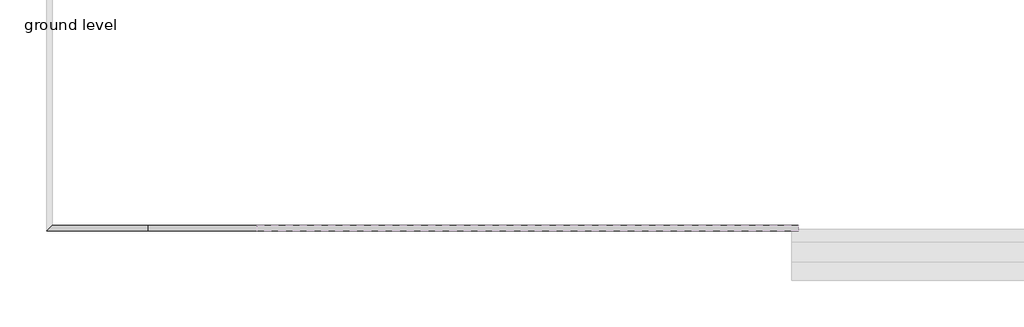
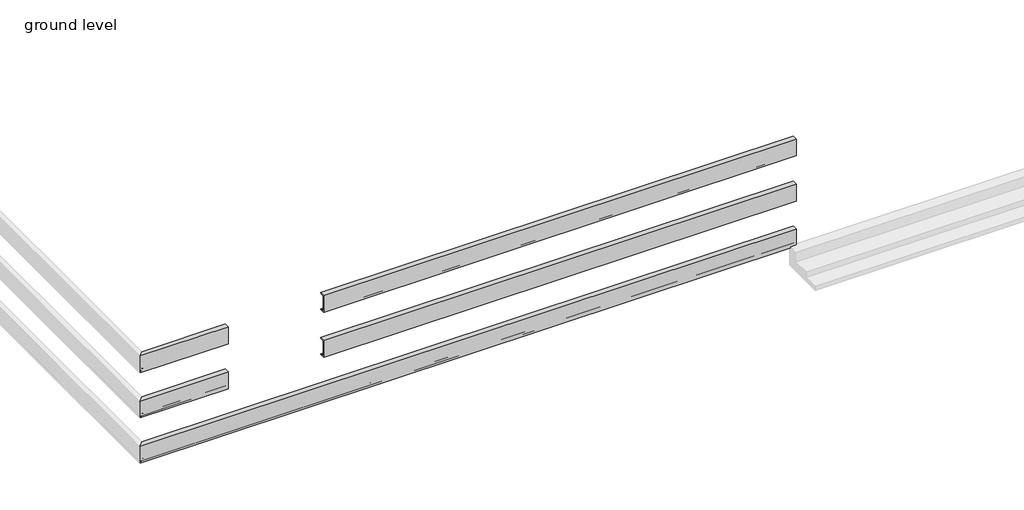
# One storey, part 1 of 3: 3 proxies.
"""IFC4 building model written with IfcOpenShell, lengths in millimetres."""

from ifc_helpers import new_model, si_unit, frame, origin, place, context, project, spatial, polyline, circle_curve, ellipse_curve, element, save
from ifc_brep_helpers import plane_surface, cylinder_surface, revolved_surface, advanced_brep

model = new_model("IFC4")

# Units and contexts
model_context = context("Model", 3, world=origin())
ifc_project = project(units=[si_unit("LENGTHUNIT", "METRE", prefix="MILLI")], contexts=[model_context])

# Site, building, storey
site = spatial("IfcSite", under=ifc_project)
building = spatial("IfcBuilding", under=site)
storey = spatial("IfcBuildingStorey", under=building, Name="ground level", Elevation=0.0)

# Proxies
placement = place(None, origin())
element("IfcBuildingElementProxy", 1, Name="Reveal", ObjectType="Reveal", at=placement, inside=storey, context=model_context, shape_type="AdvancedBrep", body=[
    advanced_brep(
    [(-10842.2672301, -7280.1146427, 1689.1), (-10842.2672301, -7216.8686427, 1689.1), (-10842.2672301, -7216.8686427, 1687.7203242), (-10842.2672301, -7221.2514519, 1682.5465897), (-10842.2672301, -7244.8721427, 1678.6098), (-10842.2672301, -7264.1100243, 1675.40348), (-10842.2672301, -7272.8756427, 1665.056011), (-10842.2672301, -7272.8756427, 1484.543989), (-10842.2672301, -7264.1100243, 1474.19652), (-10842.2672301, -7244.8721427, 1470.9902), (-10842.2672301, -7221.2514519, 1467.0534103), (-10842.2672301, -7216.8686427, 1461.8796758), (-10842.2672301, -7216.8686427, 1460.5), (-10842.2672301, -7280.1146427, 1460.5), (-4797.0672301, -7280.1146427, 1689.1), (-4797.0672301, -7280.1146427, 1460.5), (-4797.0672301, -7216.8686427, 1460.5), (-4797.0672301, -7216.8686427, 1461.8796758), (-4797.0672301, -7221.2514519, 1467.0534103), (-4797.0672301, -7244.8721427, 1470.9902), (-4797.0672301, -7264.1100243, 1474.19652), (-4797.0672301, -7272.8756427, 1484.543989), (-4797.0672301, -7272.8756427, 1665.056011), (-4797.0672301, -7264.1100243, 1675.40348), (-4797.0672301, -7244.8721427, 1678.6098), (-4797.0672301, -7221.2514519, 1682.5465897), (-4797.0672301, -7216.8686427, 1687.7203242), (-4797.0672301, -7216.8686427, 1689.1)],
    [
        (0, 1),
        (1, 2),
        (2, 3, circle_curve(frame((-10842.2672301, -7222.1137427, 1687.7203242), z_axis=(-1.0, 0.0, 0.0), x_axis=(0.0, 1.0, 0.0)), 5.2451)),
        (3, 4),
        (4, 5),
        (5, 6, circle_curve(frame((-10842.2672301, -7262.3854427, 1665.056011), z_axis=(1.0, 0.0, 0.0), x_axis=(0.0, 1.0, 0.0)), 10.4902)),
        (6, 7),
        (7, 8, circle_curve(frame((-10842.2672301, -7262.3854427, 1484.543989), z_axis=(1.0, 0.0, 0.0), x_axis=(0.0, 1.0, 0.0)), 10.4902)),
        (8, 9),
        (9, 10),
        (10, 11, circle_curve(frame((-10842.2672301, -7222.1137427, 1461.8796758), z_axis=(-1.0, 0.0, 0.0), x_axis=(0.0, 1.0, 0.0)), 5.2451)),
        (11, 12),
        (12, 13),
        (13, 0),
        (14, 15),
        (15, 16),
        (16, 17),
        (17, 18, circle_curve(frame((-4797.0672301, -7222.1137427, 1461.8796758), z_axis=(1.0, 0.0, 0.0), x_axis=(0.0, 1.0, 0.0)), 5.2451)),
        (18, 19),
        (19, 20),
        (20, 21, circle_curve(frame((-4797.0672301, -7262.3854427, 1484.543989), z_axis=(-1.0, 0.0, 0.0), x_axis=(0.0, 1.0, 0.0)), 10.4902)),
        (21, 22),
        (22, 23, circle_curve(frame((-4797.0672301, -7262.3854427, 1665.056011), z_axis=(-1.0, 0.0, 0.0), x_axis=(0.0, 1.0, 0.0)), 10.4902)),
        (23, 24),
        (24, 25),
        (25, 26, circle_curve(frame((-4797.0672301, -7222.1137427, 1687.7203242), z_axis=(1.0, 0.0, 0.0), x_axis=(0.0, 1.0, 0.0)), 5.2451)),
        (26, 27),
        (27, 14),
        (0, 14),
        (27, 1),
        (26, 2),
        (25, 3),
        (24, 4),
        (23, 5),
        (22, 6),
        (21, 7),
        (20, 8),
        (19, 9),
        (18, 10),
        (17, 11),
        (16, 12),
        (15, 13),
    ],
    [
        plane_surface(frame((-10842.2672301, -7036.6302427, 914.4), z_axis=(-1.0, 0.0, 0.0), x_axis=(0.0, -1.0, 0.0))),
        plane_surface(frame((-4797.0672301, -7265.2302427, 1450.6898298), z_axis=(1.0, 0.0, 0.0), x_axis=(0.0, 1.0, 0.0))),
        plane_surface(frame((-10842.2672301, -7280.1146427, 1689.1), z_axis=(0.0, 0.0, 1.0), x_axis=(1.0, 0.0, 0.0))),
        plane_surface(frame((-10842.2672301, -7216.8686427, 1689.1), z_axis=(0.0, 1.0, 0.0), x_axis=(1.0, 0.0, 0.0))),
        cylinder_surface(frame((-10842.2672301, -7222.1137427, 1687.7203242), z_axis=(-1.0, 0.0, 0.0), x_axis=(0.0, 1.0, 0.0)), 5.2451),
        plane_surface(frame((-10842.2672301, -7221.2514519, 1682.5465897), z_axis=(0.0, 0.16439930721687082, -0.9863938705135049), x_axis=(1.0, 0.0, 0.0))),
        plane_surface(frame((-10842.2672301, -7244.8721427, 1678.6098), z_axis=(0.0, 0.16439930721687146, -0.9863938705135048), x_axis=(1.0, 0.0, 0.0))),
        revolved_surface(polyline([(-4797.0672301, -7251.8952426999995, 1665.056011), (-10842.2672301, -7251.8952426999995, 1665.056011)]), (-10842.2672301, -7262.3854427, 1665.056011), (1.0, 0.0, 0.0)),
        plane_surface(frame((-10842.2672301, -7272.8756427, 1665.056011), z_axis=(0.0, 1.0, 0.0), x_axis=(1.0, 0.0, 0.0))),
        revolved_surface(polyline([(-4797.0672301, -7251.8952426999995, 1484.543989), (-10842.2672301, -7251.8952426999995, 1484.543989)]), (-10842.2672301, -7262.3854427, 1484.543989), (1.0, 0.0, 0.0)),
        plane_surface(frame((-10842.2672301, -7264.1100243, 1474.19652), z_axis=(0.0, 0.1643993072168769, 0.9863938705135039), x_axis=(1.0, 0.0, 0.0))),
        plane_surface(frame((-10842.2672301, -7244.8721427, 1470.9902), z_axis=(0.0, 0.16439930721687793, 0.9863938705135037), x_axis=(1.0, 0.0, 0.0))),
        cylinder_surface(frame((-10842.2672301, -7222.1137427, 1461.8796758), z_axis=(-1.0, 0.0, 0.0), x_axis=(0.0, 1.0, 0.0)), 5.2451),
        plane_surface(frame((-10842.2672301, -7216.8686427, 1461.8796758), z_axis=(0.0, 1.0, 0.0), x_axis=(1.0, 0.0, 0.0))),
        plane_surface(frame((-10842.2672301, -7216.8686427, 1460.5), z_axis=(0.0, 0.0, -1.0), x_axis=(1.0, 0.0, 0.0))),
        plane_surface(frame((-10842.2672301, -7280.1146427, 1460.5), z_axis=(0.0, -1.0, 0.0), x_axis=(1.0, 0.0, 0.0))),
    ],
    [
        (0, [[1, 2, 3, 4, 5, 6, 7, 8, 9, 10, 11, 12, 13, 14]]),
        (1, [[15, 16, 17, 18, 19, 20, 21, 22, 23, 24, 25, 26, 27, 28]]),
        (2, [[-1, 29, -28, 30]]),
        (3, [[-2, -30, -27, 31]]),
        (4, [[-3, -31, -26, 32]]),
        (5, [[-4, -32, -25, 33]]),
        (6, [[-5, -33, -24, 34]]),
        (7, [[-6, -34, -23, 35]]),
        (8, [[-7, -35, -22, 36]]),
        (9, [[-8, -36, -21, 37]]),
        (10, [[-9, -37, -20, 38]]),
        (11, [[-10, -38, -19, 39]]),
        (12, [[-11, -39, -18, 40]]),
        (13, [[-12, -40, -17, 41]]),
        (14, [[-13, -41, -16, 42]]),
        (15, [[-14, -42, -15, -29]]),
    ],
),
    advanced_brep(
    [(-13193.9516301, -7280.1146427, 1689.1), (-13130.7056301, -7216.8686427, 1689.1), (-13130.7056301, -7216.8686427, 1687.7203242), (-13135.0884393, -7221.2514519, 1682.5465897), (-13158.7091301, -7244.8721427, 1678.6098), (-13177.9470117, -7264.1100243, 1675.40348), (-13186.7126301, -7272.8756427, 1665.056011), (-13186.7126301, -7272.8756427, 1484.543989), (-13177.9470117, -7264.1100243, 1474.19652), (-13158.7091301, -7244.8721427, 1470.9902), (-13135.0884393, -7221.2514519, 1467.0534103), (-13130.7056301, -7216.8686427, 1461.8796758), (-13130.7056301, -7216.8686427, 1460.5), (-13193.9516301, -7280.1146427, 1460.5), (-12061.4672301, -7280.1146427, 1689.1), (-12061.4672301, -7280.1146427, 1460.5), (-12061.4672301, -7216.8686427, 1460.5), (-12061.4672301, -7216.8686427, 1461.8796758), (-12061.4672301, -7221.2514519, 1467.0534103), (-12061.4672301, -7244.8721427, 1470.9902), (-12061.4672301, -7264.1100243, 1474.19652), (-12061.4672301, -7272.8756427, 1484.543989), (-12061.4672301, -7272.8756427, 1665.056011), (-12061.4672301, -7264.1100243, 1675.40348), (-12061.4672301, -7244.8721427, 1678.6098), (-12061.4672301, -7221.2514519, 1682.5465897), (-12061.4672301, -7216.8686427, 1687.7203242), (-12061.4672301, -7216.8686427, 1689.1)],
    [
        (0, 1),
        (1, 2),
        (2, 3, ellipse_curve(frame((-13135.9507301, -7222.1137427, 1687.7203242), z_axis=(-0.7071067811865476, 0.7071067811865476, 0.0), x_axis=(-0.7071067811865475, -0.7071067811865476, 0.0)), 7.4176916, 5.2451)),
        (3, 4),
        (4, 5),
        (5, 6, ellipse_curve(frame((-13176.2224301, -7262.3854427, 1665.056011), z_axis=(0.7071067811865476, -0.7071067811865476, 0.0), x_axis=(0.7071067811865475, 0.7071067811865476, 0.0)), 14.8353831, 10.4902)),
        (6, 7),
        (7, 8, ellipse_curve(frame((-13176.2224301, -7262.3854427, 1484.543989), z_axis=(0.7071067811865476, -0.7071067811865476, 0.0), x_axis=(0.7071067811865475, 0.7071067811865476, 0.0)), 14.8353831, 10.4902)),
        (8, 9),
        (9, 10),
        (10, 11, ellipse_curve(frame((-13135.9507301, -7222.1137427, 1461.8796758), z_axis=(-0.7071067811865476, 0.7071067811865476, 0.0), x_axis=(-0.7071067811865475, -0.7071067811865476, 0.0)), 7.4176916, 5.2451)),
        (11, 12),
        (12, 13),
        (13, 0),
        (14, 15),
        (15, 16),
        (16, 17),
        (17, 18, circle_curve(frame((-12061.4672301, -7222.1137427, 1461.8796758), z_axis=(1.0, 0.0, 0.0), x_axis=(0.0, 1.0, 0.0)), 5.2451)),
        (18, 19),
        (19, 20),
        (20, 21, circle_curve(frame((-12061.4672301, -7262.3854427, 1484.543989), z_axis=(-1.0, 0.0, 0.0), x_axis=(0.0, 1.0, 0.0)), 10.4902)),
        (21, 22),
        (22, 23, circle_curve(frame((-12061.4672301, -7262.3854427, 1665.056011), z_axis=(-1.0, 0.0, 0.0), x_axis=(0.0, 1.0, 0.0)), 10.4902)),
        (23, 24),
        (24, 25),
        (25, 26, circle_curve(frame((-12061.4672301, -7222.1137427, 1687.7203242), z_axis=(1.0, 0.0, 0.0), x_axis=(0.0, 1.0, 0.0)), 5.2451)),
        (26, 27),
        (27, 14),
        (0, 14),
        (27, 1),
        (26, 2),
        (25, 3),
        (24, 4),
        (23, 5),
        (22, 6),
        (21, 7),
        (20, 8),
        (19, 9),
        (18, 10),
        (17, 11),
        (16, 12),
        (15, 13),
    ],
    [
        plane_surface(frame((-13179.0672301, -7265.2302427, 1270.0), z_axis=(-0.7071067811865476, 0.7071067811865476, 0.0), x_axis=(0.7071067811865476, 0.7071067811865476, 0.0))),
        plane_surface(frame((-12061.4672301, -7036.6302427, 2184.4), z_axis=(1.0, 0.0, 0.0), x_axis=(0.0, -1.0, 0.0))),
        plane_surface(frame((-13193.9516301, -7280.1146427, 1689.1), z_axis=(0.0, 0.0, 1.0), x_axis=(1.0, 0.0, 0.0))),
        plane_surface(frame((-13130.7056301, -7216.8686427, 1689.1), z_axis=(0.0, 1.0, 0.0), x_axis=(1.0, 0.0, 0.0))),
        cylinder_surface(frame((-13179.0672301, -7222.1137427, 1687.7203242), z_axis=(-1.0, 0.0, 0.0), x_axis=(0.0, 1.0, 0.0)), 5.2451),
        plane_surface(frame((-13135.0884393, -7221.2514519, 1682.5465897), z_axis=(0.0, 0.16439930721687082, -0.9863938705135049), x_axis=(1.0, 0.0, 0.0))),
        plane_surface(frame((-13158.7091301, -7244.8721427, 1678.6098), z_axis=(0.0, 0.16439930721687146, -0.9863938705135048), x_axis=(1.0, 0.0, 0.0))),
        revolved_surface(polyline([(-12061.4672301, -7251.8952426999995, 1665.056011), (-13186.7126301, -7251.8952426999995, 1665.056011)]), (-13179.0672301, -7262.3854427, 1665.056011), (1.0, 0.0, 0.0)),
        plane_surface(frame((-13186.7126301, -7272.8756427, 1665.056011), z_axis=(0.0, 1.0, 0.0), x_axis=(1.0, 0.0, 0.0))),
        revolved_surface(polyline([(-12061.4672301, -7251.8952426999995, 1484.543989), (-13186.7126301, -7251.8952426999995, 1484.543989)]), (-13179.0672301, -7262.3854427, 1484.543989), (1.0, 0.0, 0.0)),
        plane_surface(frame((-13177.9470117, -7264.1100243, 1474.19652), z_axis=(0.0, 0.1643993072168769, 0.9863938705135039), x_axis=(1.0, 0.0, 0.0))),
        plane_surface(frame((-13158.7091301, -7244.8721427, 1470.9902), z_axis=(0.0, 0.16439930721687793, 0.9863938705135037), x_axis=(1.0, 0.0, 0.0))),
        cylinder_surface(frame((-13179.0672301, -7222.1137427, 1461.8796758), z_axis=(-1.0, 0.0, 0.0), x_axis=(0.0, 1.0, 0.0)), 5.2451),
        plane_surface(frame((-13130.7056301, -7216.8686427, 1461.8796758), z_axis=(0.0, 1.0, 0.0), x_axis=(1.0, 0.0, 0.0))),
        plane_surface(frame((-13130.7056301, -7216.8686427, 1460.5), z_axis=(0.0, 0.0, -1.0), x_axis=(1.0, 0.0, 0.0))),
        plane_surface(frame((-13193.9516301, -7280.1146427, 1460.5), z_axis=(0.0, -1.0, 0.0), x_axis=(1.0, 0.0, 0.0))),
    ],
    [
        (0, [[1, 2, 3, 4, 5, 6, 7, 8, 9, 10, 11, 12, 13, 14]]),
        (1, [[15, 16, 17, 18, 19, 20, 21, 22, 23, 24, 25, 26, 27, 28]]),
        (2, [[-1, 29, -28, 30]]),
        (3, [[-2, -30, -27, 31]]),
        (4, [[-3, -31, -26, 32]]),
        (5, [[-4, -32, -25, 33]]),
        (6, [[-5, -33, -24, 34]]),
        (7, [[-6, -34, -23, 35]]),
        (8, [[-7, -35, -22, 36]]),
        (9, [[-8, -36, -21, 37]]),
        (10, [[-9, -37, -20, 38]]),
        (11, [[-10, -38, -19, 39]]),
        (12, [[-11, -39, -18, 40]]),
        (13, [[-12, -40, -17, 41]]),
        (14, [[-13, -41, -16, 42]]),
        (15, [[-14, -42, -15, -29]]),
    ],
),
])
element("IfcBuildingElementProxy", 2, Name="Reveal", ObjectType="Reveal", at=placement, inside=storey, context=model_context, shape_type="AdvancedBrep", body=[
    advanced_brep(
    [(-10842.2672301, -7280.1146427, 1079.5), (-10842.2672301, -7216.8686427, 1079.5), (-10842.2672301, -7216.8686427, 1078.1203242), (-10842.2672301, -7221.2514519, 1072.9465897), (-10842.2672301, -7244.8721427, 1069.0098), (-10842.2672301, -7264.1100243, 1065.80348), (-10842.2672301, -7272.8756427, 1055.456011), (-10842.2672301, -7272.8756427, 874.943989), (-10842.2672301, -7264.1100243, 864.59652), (-10842.2672301, -7244.8721427, 861.3902), (-10842.2672301, -7221.2514519, 857.4534103), (-10842.2672301, -7216.8686427, 852.2796758), (-10842.2672301, -7216.8686427, 850.9), (-10842.2672301, -7280.1146427, 850.9), (-4797.0672301, -7280.1146427, 1079.5), (-4797.0672301, -7280.1146427, 850.9), (-4797.0672301, -7216.8686427, 850.9), (-4797.0672301, -7216.8686427, 852.2796758), (-4797.0672301, -7221.2514519, 857.4534103), (-4797.0672301, -7244.8721427, 861.3902), (-4797.0672301, -7264.1100243, 864.59652), (-4797.0672301, -7272.8756427, 874.943989), (-4797.0672301, -7272.8756427, 1055.456011), (-4797.0672301, -7264.1100243, 1065.80348), (-4797.0672301, -7244.8721427, 1069.0098), (-4797.0672301, -7221.2514519, 1072.9465897), (-4797.0672301, -7216.8686427, 1078.1203242), (-4797.0672301, -7216.8686427, 1079.5)],
    [
        (0, 1),
        (1, 2),
        (2, 3, circle_curve(frame((-10842.2672301, -7222.1137427, 1078.1203242), z_axis=(-1.0, 0.0, 0.0), x_axis=(0.0, 1.0, 0.0)), 5.2451)),
        (3, 4),
        (4, 5),
        (5, 6, circle_curve(frame((-10842.2672301, -7262.3854427, 1055.456011), z_axis=(1.0, 0.0, 0.0), x_axis=(0.0, 1.0, 0.0)), 10.4902)),
        (6, 7),
        (7, 8, circle_curve(frame((-10842.2672301, -7262.3854427, 874.943989), z_axis=(1.0, 0.0, 0.0), x_axis=(0.0, 1.0, 0.0)), 10.4902)),
        (8, 9),
        (9, 10),
        (10, 11, circle_curve(frame((-10842.2672301, -7222.1137427, 852.2796758), z_axis=(-1.0, 0.0, 0.0), x_axis=(0.0, 1.0, 0.0)), 5.2451)),
        (11, 12),
        (12, 13),
        (13, 0),
        (14, 15),
        (15, 16),
        (16, 17),
        (17, 18, circle_curve(frame((-4797.0672301, -7222.1137427, 852.2796758), z_axis=(1.0, 0.0, 0.0), x_axis=(0.0, 1.0, 0.0)), 5.2451)),
        (18, 19),
        (19, 20),
        (20, 21, circle_curve(frame((-4797.0672301, -7262.3854427, 874.943989), z_axis=(-1.0, 0.0, 0.0), x_axis=(0.0, 1.0, 0.0)), 10.4902)),
        (21, 22),
        (22, 23, circle_curve(frame((-4797.0672301, -7262.3854427, 1055.456011), z_axis=(-1.0, 0.0, 0.0), x_axis=(0.0, 1.0, 0.0)), 10.4902)),
        (23, 24),
        (24, 25),
        (25, 26, circle_curve(frame((-4797.0672301, -7222.1137427, 1078.1203242), z_axis=(1.0, 0.0, 0.0), x_axis=(0.0, 1.0, 0.0)), 5.2451)),
        (26, 27),
        (27, 14),
        (0, 14),
        (27, 1),
        (26, 2),
        (25, 3),
        (24, 4),
        (23, 5),
        (22, 6),
        (21, 7),
        (20, 8),
        (19, 9),
        (18, 10),
        (17, 11),
        (16, 12),
        (15, 13),
    ],
    [
        plane_surface(frame((-10842.2672301, -7036.6302427, 914.4), z_axis=(-1.0, 0.0, 0.0), x_axis=(0.0, -1.0, 0.0))),
        plane_surface(frame((-4797.0672301, -7265.2302427, 841.0898298), z_axis=(1.0, 0.0, 0.0), x_axis=(0.0, 1.0, 0.0))),
        plane_surface(frame((-10842.2672301, -7280.1146427, 1079.5), z_axis=(0.0, 0.0, 1.0), x_axis=(1.0, 0.0, 0.0))),
        plane_surface(frame((-10842.2672301, -7216.8686427, 1079.5), z_axis=(0.0, 1.0, 0.0), x_axis=(1.0, 0.0, 0.0))),
        cylinder_surface(frame((-10842.2672301, -7222.1137427, 1078.1203242), z_axis=(-1.0, 0.0, 0.0), x_axis=(0.0, 1.0, 0.0)), 5.2451),
        plane_surface(frame((-10842.2672301, -7221.2514519, 1072.9465897), z_axis=(0.0, 0.16439930721687082, -0.9863938705135049), x_axis=(1.0, 0.0, 0.0))),
        plane_surface(frame((-10842.2672301, -7244.8721427, 1069.0098), z_axis=(0.0, 0.16439930721687146, -0.9863938705135048), x_axis=(1.0, 0.0, 0.0))),
        revolved_surface(polyline([(-4797.0672301, -7251.8952426999995, 1055.456011), (-10842.2672301, -7251.8952426999995, 1055.456011)]), (-10842.2672301, -7262.3854427, 1055.456011), (1.0, 0.0, 0.0)),
        plane_surface(frame((-10842.2672301, -7272.8756427, 1055.456011), z_axis=(0.0, 1.0, 0.0), x_axis=(1.0, 0.0, 0.0))),
        revolved_surface(polyline([(-4797.0672301, -7251.8952426999995, 874.943989), (-10842.2672301, -7251.8952426999995, 874.943989)]), (-10842.2672301, -7262.3854427, 874.943989), (1.0, 0.0, 0.0)),
        plane_surface(frame((-10842.2672301, -7264.1100243, 864.59652), z_axis=(0.0, 0.1643993072168769, 0.9863938705135039), x_axis=(1.0, 0.0, 0.0))),
        plane_surface(frame((-10842.2672301, -7244.8721427, 861.3902), z_axis=(0.0, 0.16439930721687793, 0.9863938705135037), x_axis=(1.0, 0.0, 0.0))),
        cylinder_surface(frame((-10842.2672301, -7222.1137427, 852.2796758), z_axis=(-1.0, 0.0, 0.0), x_axis=(0.0, 1.0, 0.0)), 5.2451),
        plane_surface(frame((-10842.2672301, -7216.8686427, 852.2796758), z_axis=(0.0, 1.0, 0.0), x_axis=(1.0, 0.0, 0.0))),
        plane_surface(frame((-10842.2672301, -7216.8686427, 850.9), z_axis=(0.0, 0.0, -1.0), x_axis=(1.0, 0.0, 0.0))),
        plane_surface(frame((-10842.2672301, -7280.1146427, 850.9), z_axis=(0.0, -1.0, 0.0), x_axis=(1.0, 0.0, 0.0))),
    ],
    [
        (0, [[1, 2, 3, 4, 5, 6, 7, 8, 9, 10, 11, 12, 13, 14]]),
        (1, [[15, 16, 17, 18, 19, 20, 21, 22, 23, 24, 25, 26, 27, 28]]),
        (2, [[-1, 29, -28, 30]]),
        (3, [[-2, -30, -27, 31]]),
        (4, [[-3, -31, -26, 32]]),
        (5, [[-4, -32, -25, 33]]),
        (6, [[-5, -33, -24, 34]]),
        (7, [[-6, -34, -23, 35]]),
        (8, [[-7, -35, -22, 36]]),
        (9, [[-8, -36, -21, 37]]),
        (10, [[-9, -37, -20, 38]]),
        (11, [[-10, -38, -19, 39]]),
        (12, [[-11, -39, -18, 40]]),
        (13, [[-12, -40, -17, 41]]),
        (14, [[-13, -41, -16, 42]]),
        (15, [[-14, -42, -15, -29]]),
    ],
),
    advanced_brep(
    [(-13193.9516301, -7280.1146427, 1079.5), (-13130.7056301, -7216.8686427, 1079.5), (-13130.7056301, -7216.8686427, 1078.1203242), (-13135.0884393, -7221.2514519, 1072.9465897), (-13158.7091301, -7244.8721427, 1069.0098), (-13177.9470117, -7264.1100243, 1065.80348), (-13186.7126301, -7272.8756427, 1055.456011), (-13186.7126301, -7272.8756427, 874.943989), (-13177.9470117, -7264.1100243, 864.59652), (-13158.7091301, -7244.8721427, 861.3902), (-13135.0884393, -7221.2514519, 857.4534103), (-13130.7056301, -7216.8686427, 852.2796758), (-13130.7056301, -7216.8686427, 850.9), (-13193.9516301, -7280.1146427, 850.9), (-12061.4672301, -7280.1146427, 1079.5), (-12061.4672301, -7280.1146427, 850.9), (-12061.4672301, -7216.8686427, 850.9), (-12061.4672301, -7216.8686427, 852.2796758), (-12061.4672301, -7221.2514519, 857.4534103), (-12061.4672301, -7244.8721427, 861.3902), (-12061.4672301, -7264.1100243, 864.59652), (-12061.4672301, -7272.8756427, 874.943989), (-12061.4672301, -7272.8756427, 1055.456011), (-12061.4672301, -7264.1100243, 1065.80348), (-12061.4672301, -7244.8721427, 1069.0098), (-12061.4672301, -7221.2514519, 1072.9465897), (-12061.4672301, -7216.8686427, 1078.1203242), (-12061.4672301, -7216.8686427, 1079.5)],
    [
        (0, 1),
        (1, 2),
        (2, 3, ellipse_curve(frame((-13135.9507301, -7222.1137427, 1078.1203242), z_axis=(-0.7071067811865476, 0.7071067811865476, 0.0), x_axis=(-0.7071067811865475, -0.7071067811865476, 0.0)), 7.4176916, 5.2451)),
        (3, 4),
        (4, 5),
        (5, 6, ellipse_curve(frame((-13176.2224301, -7262.3854427, 1055.456011), z_axis=(0.7071067811865476, -0.7071067811865476, 0.0), x_axis=(0.7071067811865475, 0.7071067811865476, 0.0)), 14.8353831, 10.4902)),
        (6, 7),
        (7, 8, ellipse_curve(frame((-13176.2224301, -7262.3854427, 874.943989), z_axis=(0.7071067811865476, -0.7071067811865476, 0.0), x_axis=(0.7071067811865475, 0.7071067811865476, 0.0)), 14.8353831, 10.4902)),
        (8, 9),
        (9, 10),
        (10, 11, ellipse_curve(frame((-13135.9507301, -7222.1137427, 852.2796758), z_axis=(-0.7071067811865476, 0.7071067811865476, 0.0), x_axis=(-0.7071067811865475, -0.7071067811865476, 0.0)), 7.4176916, 5.2451)),
        (11, 12),
        (12, 13),
        (13, 0),
        (14, 15),
        (15, 16),
        (16, 17),
        (17, 18, circle_curve(frame((-12061.4672301, -7222.1137427, 852.2796758), z_axis=(1.0, 0.0, 0.0), x_axis=(0.0, 1.0, 0.0)), 5.2451)),
        (18, 19),
        (19, 20),
        (20, 21, circle_curve(frame((-12061.4672301, -7262.3854427, 874.943989), z_axis=(-1.0, 0.0, 0.0), x_axis=(0.0, 1.0, 0.0)), 10.4902)),
        (21, 22),
        (22, 23, circle_curve(frame((-12061.4672301, -7262.3854427, 1055.456011), z_axis=(-1.0, 0.0, 0.0), x_axis=(0.0, 1.0, 0.0)), 10.4902)),
        (23, 24),
        (24, 25),
        (25, 26, circle_curve(frame((-12061.4672301, -7222.1137427, 1078.1203242), z_axis=(1.0, 0.0, 0.0), x_axis=(0.0, 1.0, 0.0)), 5.2451)),
        (26, 27),
        (27, 14),
        (0, 14),
        (27, 1),
        (26, 2),
        (25, 3),
        (24, 4),
        (23, 5),
        (22, 6),
        (21, 7),
        (20, 8),
        (19, 9),
        (18, 10),
        (17, 11),
        (16, 12),
        (15, 13),
    ],
    [
        plane_surface(frame((-13179.0672301, -7265.2302427, 660.4), z_axis=(-0.7071067811865476, 0.7071067811865476, 0.0), x_axis=(0.7071067811865476, 0.7071067811865476, 0.0))),
        plane_surface(frame((-12061.4672301, -7036.6302427, 2184.4), z_axis=(1.0, 0.0, 0.0), x_axis=(0.0, -1.0, 0.0))),
        plane_surface(frame((-13193.9516301, -7280.1146427, 1079.5), z_axis=(0.0, 0.0, 1.0), x_axis=(1.0, 0.0, 0.0))),
        plane_surface(frame((-13130.7056301, -7216.8686427, 1079.5), z_axis=(0.0, 1.0, 0.0), x_axis=(1.0, 0.0, 0.0))),
        cylinder_surface(frame((-13179.0672301, -7222.1137427, 1078.1203242), z_axis=(-1.0, 0.0, 0.0), x_axis=(0.0, 1.0, 0.0)), 5.2451),
        plane_surface(frame((-13135.0884393, -7221.2514519, 1072.9465897), z_axis=(0.0, 0.16439930721687082, -0.9863938705135049), x_axis=(1.0, 0.0, 0.0))),
        plane_surface(frame((-13158.7091301, -7244.8721427, 1069.0098), z_axis=(0.0, 0.16439930721687146, -0.9863938705135048), x_axis=(1.0, 0.0, 0.0))),
        revolved_surface(polyline([(-12061.4672301, -7251.8952426999995, 1055.456011), (-13186.7126301, -7251.8952426999995, 1055.456011)]), (-13179.0672301, -7262.3854427, 1055.456011), (1.0, 0.0, 0.0)),
        plane_surface(frame((-13186.7126301, -7272.8756427, 1055.456011), z_axis=(0.0, 1.0, 0.0), x_axis=(1.0, 0.0, 0.0))),
        revolved_surface(polyline([(-12061.4672301, -7251.8952426999995, 874.943989), (-13186.7126301, -7251.8952426999995, 874.943989)]), (-13179.0672301, -7262.3854427, 874.943989), (1.0, 0.0, 0.0)),
        plane_surface(frame((-13177.9470117, -7264.1100243, 864.59652), z_axis=(0.0, 0.1643993072168769, 0.9863938705135039), x_axis=(1.0, 0.0, 0.0))),
        plane_surface(frame((-13158.7091301, -7244.8721427, 861.3902), z_axis=(0.0, 0.16439930721687793, 0.9863938705135037), x_axis=(1.0, 0.0, 0.0))),
        cylinder_surface(frame((-13179.0672301, -7222.1137427, 852.2796758), z_axis=(-1.0, 0.0, 0.0), x_axis=(0.0, 1.0, 0.0)), 5.2451),
        plane_surface(frame((-13130.7056301, -7216.8686427, 852.2796758), z_axis=(0.0, 1.0, 0.0), x_axis=(1.0, 0.0, 0.0))),
        plane_surface(frame((-13130.7056301, -7216.8686427, 850.9), z_axis=(0.0, 0.0, -1.0), x_axis=(1.0, 0.0, 0.0))),
        plane_surface(frame((-13193.9516301, -7280.1146427, 850.9), z_axis=(0.0, -1.0, 0.0), x_axis=(1.0, 0.0, 0.0))),
    ],
    [
        (0, [[1, 2, 3, 4, 5, 6, 7, 8, 9, 10, 11, 12, 13, 14]]),
        (1, [[15, 16, 17, 18, 19, 20, 21, 22, 23, 24, 25, 26, 27, 28]]),
        (2, [[-1, 29, -28, 30]]),
        (3, [[-2, -30, -27, 31]]),
        (4, [[-3, -31, -26, 32]]),
        (5, [[-4, -32, -25, 33]]),
        (6, [[-5, -33, -24, 34]]),
        (7, [[-6, -34, -23, 35]]),
        (8, [[-7, -35, -22, 36]]),
        (9, [[-8, -36, -21, 37]]),
        (10, [[-9, -37, -20, 38]]),
        (11, [[-10, -38, -19, 39]]),
        (12, [[-11, -39, -18, 40]]),
        (13, [[-12, -40, -17, 41]]),
        (14, [[-13, -41, -16, 42]]),
        (15, [[-14, -42, -15, -29]]),
    ],
),
])
element("IfcBuildingElementProxy", 3, Name="Reveal", ObjectType="Reveal", at=placement, inside=storey, context=model_context, shape_type="AdvancedBrep", body=[
    advanced_brep(
    [(-13193.9516301, -7280.1146427, 469.9), (-13130.7056301, -7216.8686427, 469.9), (-13130.7056301, -7216.8686427, 468.5203242), (-13135.0884393, -7221.2514519, 463.3465897), (-13158.7091301, -7244.8721427, 459.4098), (-13177.9470117, -7264.1100243, 456.20348), (-13186.7126301, -7272.8756427, 445.856011), (-13186.7126301, -7272.8756427, 265.343989), (-13177.9470117, -7264.1100243, 254.99652), (-13158.7091301, -7244.8721427, 251.7902), (-13135.0884393, -7221.2514519, 247.8534103), (-13130.7056301, -7216.8686427, 242.6796758), (-13130.7056301, -7216.8686427, 241.3), (-13193.9516301, -7280.1146427, 241.3), (-4797.0672301, -7280.1146427, 469.9), (-4797.0672301, -7280.1146427, 241.3), (-4797.0672301, -7216.8686427, 241.3), (-4797.0672301, -7216.8686427, 242.6796758), (-4797.0672301, -7221.2514519, 247.8534103), (-4797.0672301, -7244.8721427, 251.7902), (-4797.0672301, -7264.1100243, 254.99652), (-4797.0672301, -7272.8756427, 265.343989), (-4797.0672301, -7272.8756427, 445.856011), (-4797.0672301, -7264.1100243, 456.20348), (-4797.0672301, -7244.8721427, 459.4098), (-4797.0672301, -7221.2514519, 463.3465897), (-4797.0672301, -7216.8686427, 468.5203242), (-4797.0672301, -7216.8686427, 469.9)],
    [
        (0, 1),
        (1, 2),
        (2, 3, ellipse_curve(frame((-13135.9507301, -7222.1137427, 468.5203242), z_axis=(-0.7071067811865476, 0.7071067811865476, 0.0), x_axis=(-0.7071067811865475, -0.7071067811865476, 0.0)), 7.4176916, 5.2451)),
        (3, 4),
        (4, 5),
        (5, 6, ellipse_curve(frame((-13176.2224301, -7262.3854427, 445.856011), z_axis=(0.7071067811865476, -0.7071067811865476, 0.0), x_axis=(0.7071067811865475, 0.7071067811865476, 0.0)), 14.8353831, 10.4902)),
        (6, 7),
        (7, 8, ellipse_curve(frame((-13176.2224301, -7262.3854427, 265.343989), z_axis=(0.7071067811865476, -0.7071067811865476, 0.0), x_axis=(0.7071067811865475, 0.7071067811865476, 0.0)), 14.8353831, 10.4902)),
        (8, 9),
        (9, 10),
        (10, 11, ellipse_curve(frame((-13135.9507301, -7222.1137427, 242.6796758), z_axis=(-0.7071067811865476, 0.7071067811865476, 0.0), x_axis=(-0.7071067811865475, -0.7071067811865476, 0.0)), 7.4176916, 5.2451)),
        (11, 12),
        (12, 13),
        (13, 0),
        (14, 15),
        (15, 16),
        (16, 17),
        (17, 18, circle_curve(frame((-4797.0672301, -7222.1137427, 242.6796758), z_axis=(1.0, 0.0, 0.0), x_axis=(0.0, 1.0, 0.0)), 5.2451)),
        (18, 19),
        (19, 20),
        (20, 21, circle_curve(frame((-4797.0672301, -7262.3854427, 265.343989), z_axis=(-1.0, 0.0, 0.0), x_axis=(0.0, 1.0, 0.0)), 10.4902)),
        (21, 22),
        (22, 23, circle_curve(frame((-4797.0672301, -7262.3854427, 445.856011), z_axis=(-1.0, 0.0, 0.0), x_axis=(0.0, 1.0, 0.0)), 10.4902)),
        (23, 24),
        (24, 25),
        (25, 26, circle_curve(frame((-4797.0672301, -7222.1137427, 468.5203242), z_axis=(1.0, 0.0, 0.0), x_axis=(0.0, 1.0, 0.0)), 5.2451)),
        (26, 27),
        (27, 14),
        (0, 14),
        (27, 1),
        (26, 2),
        (25, 3),
        (24, 4),
        (23, 5),
        (22, 6),
        (21, 7),
        (20, 8),
        (19, 9),
        (18, 10),
        (17, 11),
        (16, 12),
        (15, 13),
    ],
    [
        plane_surface(frame((-13179.0672301, -7265.2302427, 50.8), z_axis=(-0.7071067811865476, 0.7071067811865476, 0.0), x_axis=(0.7071067811865476, 0.7071067811865476, 0.0))),
        plane_surface(frame((-4797.0672301, -7265.2302427, 231.4898298), z_axis=(1.0, 0.0, 0.0), x_axis=(0.0, 1.0, 0.0))),
        plane_surface(frame((-13193.9516301, -7280.1146427, 469.9), z_axis=(0.0, 0.0, 1.0), x_axis=(1.0, 0.0, 0.0))),
        plane_surface(frame((-13130.7056301, -7216.8686427, 469.9), z_axis=(0.0, 1.0, 0.0), x_axis=(1.0, 0.0, 0.0))),
        cylinder_surface(frame((-13179.0672301, -7222.1137427, 468.5203242), z_axis=(-1.0, 0.0, 0.0), x_axis=(0.0, 1.0, 0.0)), 5.2451),
        plane_surface(frame((-13135.0884393, -7221.2514519, 463.3465897), z_axis=(0.0, 0.16439930721687082, -0.9863938705135049), x_axis=(1.0, 0.0, 0.0))),
        plane_surface(frame((-13158.7091301, -7244.8721427, 459.4098), z_axis=(0.0, 0.16439930721687146, -0.9863938705135048), x_axis=(1.0, 0.0, 0.0))),
        revolved_surface(polyline([(-4797.0672300999995, -7251.8952426999995, 445.856011), (-13186.7126301, -7251.8952426999995, 445.856011)]), (-13179.0672301, -7262.3854427, 445.856011), (1.0, 0.0, 0.0)),
        plane_surface(frame((-13186.7126301, -7272.8756427, 445.856011), z_axis=(0.0, 1.0, 0.0), x_axis=(1.0, 0.0, 0.0))),
        revolved_surface(polyline([(-4797.0672300999995, -7251.8952426999995, 265.343989), (-13186.7126301, -7251.8952426999995, 265.343989)]), (-13179.0672301, -7262.3854427, 265.343989), (1.0, 0.0, 0.0)),
        plane_surface(frame((-13177.9470117, -7264.1100243, 254.99652), z_axis=(0.0, 0.1643993072168769, 0.9863938705135039), x_axis=(1.0, 0.0, 0.0))),
        plane_surface(frame((-13158.7091301, -7244.8721427, 251.7902), z_axis=(0.0, 0.16439930721687793, 0.9863938705135037), x_axis=(1.0, 0.0, 0.0))),
        cylinder_surface(frame((-13179.0672301, -7222.1137427, 242.6796758), z_axis=(-1.0, 0.0, 0.0), x_axis=(0.0, 1.0, 0.0)), 5.2451),
        plane_surface(frame((-13130.7056301, -7216.8686427, 242.6796758), z_axis=(0.0, 1.0, 0.0), x_axis=(1.0, 0.0, 0.0))),
        plane_surface(frame((-13130.7056301, -7216.8686427, 241.3), z_axis=(0.0, 0.0, -1.0), x_axis=(1.0, 0.0, 0.0))),
        plane_surface(frame((-13193.9516301, -7280.1146427, 241.3), z_axis=(0.0, -1.0, 0.0), x_axis=(1.0, 0.0, 0.0))),
    ],
    [
        (0, [[1, 2, 3, 4, 5, 6, 7, 8, 9, 10, 11, 12, 13, 14]]),
        (1, [[15, 16, 17, 18, 19, 20, 21, 22, 23, 24, 25, 26, 27, 28]]),
        (2, [[-1, 29, -28, 30]]),
        (3, [[-2, -30, -27, 31]]),
        (4, [[-3, -31, -26, 32]]),
        (5, [[-4, -32, -25, 33]]),
        (6, [[-5, -33, -24, 34]]),
        (7, [[-6, -34, -23, 35]]),
        (8, [[-7, -35, -22, 36]]),
        (9, [[-8, -36, -21, 37]]),
        (10, [[-9, -37, -20, 38]]),
        (11, [[-10, -38, -19, 39]]),
        (12, [[-11, -39, -18, 40]]),
        (13, [[-12, -40, -17, 41]]),
        (14, [[-13, -41, -16, 42]]),
        (15, [[-14, -42, -15, -29]]),
    ],
),
])

save(model, "model.ifc")
